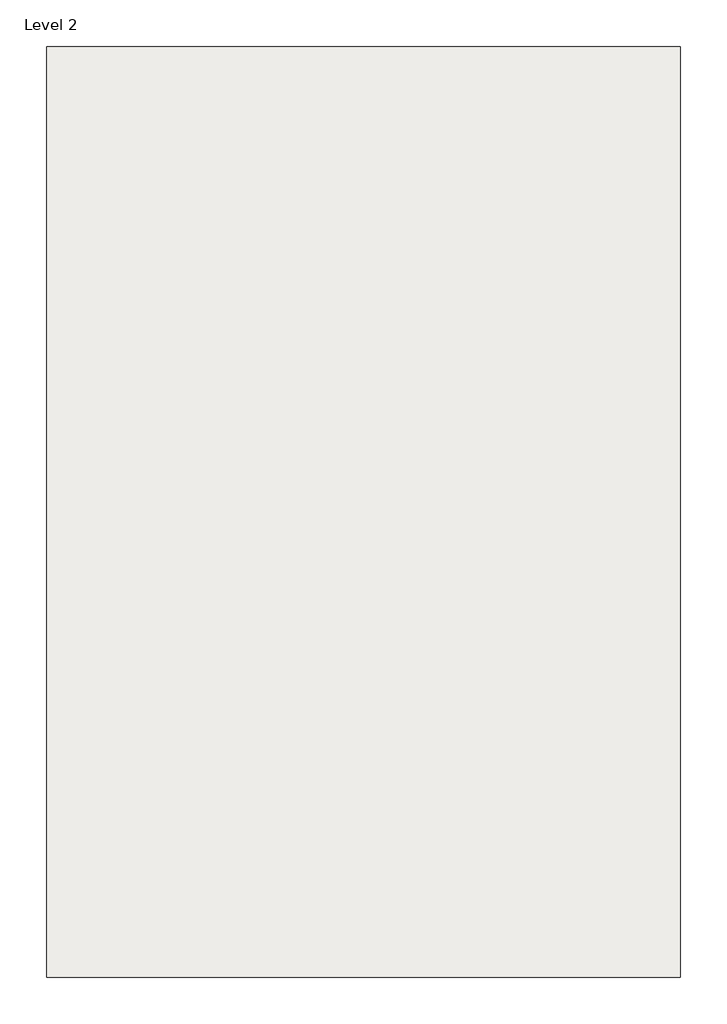
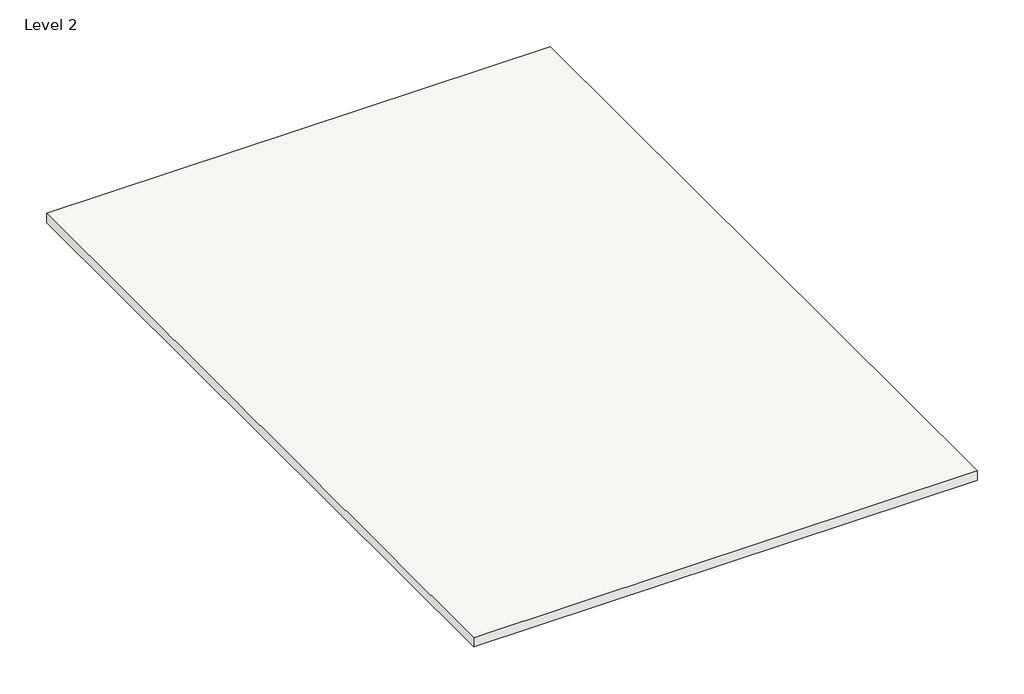
# One storey, incomplete: 1 roof.
"""IFC4 building model written with IfcOpenShell, lengths in millimetres."""

from ifc_helpers import new_model, si_unit, frame, origin, place, context, project, spatial, polyline, outline, extrude, element, save

model = new_model("IFC4")

# Units and contexts
model_context = context("Model", 3, world=origin())
ifc_project = project(units=[si_unit("LENGTHUNIT", "METRE", prefix="MILLI")], contexts=[model_context])

# Site, building, storey
site = spatial("IfcSite", under=ifc_project)
building = spatial("IfcBuilding", under=site)
storey = spatial("IfcBuildingStorey", under=building, Name="Level 2", Elevation=3048.0)

# Roof
placement = place(None, origin())
element("IfcRoof", 1, ObjectType="Generic - 12\"", at=placement, inside=storey, context=model_context, shape_type="SweptSolid", body=[
    extrude(outline(polyline([(-5216.1449167, 6076.3773594), (2670.5550833, 6076.3773594), (2670.5550833, -5508.2570853), (-5216.1449167, -5508.2570853), (-5216.1449167, 6076.3773594)])), frame((0.0, 0.0, 3048.0), z_axis=(0.0, 0.0, 1.0), x_axis=(1.0, 0.0, 0.0)), (0.0, 0.0, 1.0), 152.4),
])

save(model, "model.ifc")

# Revit data of these elements
# Type "Generic - 12\""
#   Assembly Code = "B1020"
#   Layers, outside or top first: 0' - 6" no material (function 1)
# Element 1 (IfcRoof, "Generic - 12\"")
#   built-in parameter 1001705 = 10.5 (stored number, unit not read)
#   built-in parameter 1001710 = 33615
#   Phase Created = New Construction
#   Materials on its faces: "Default Roof"
# Materials
#   "Default Roof": colour RGB 88 101 114, transparency 0, Cost = 0
